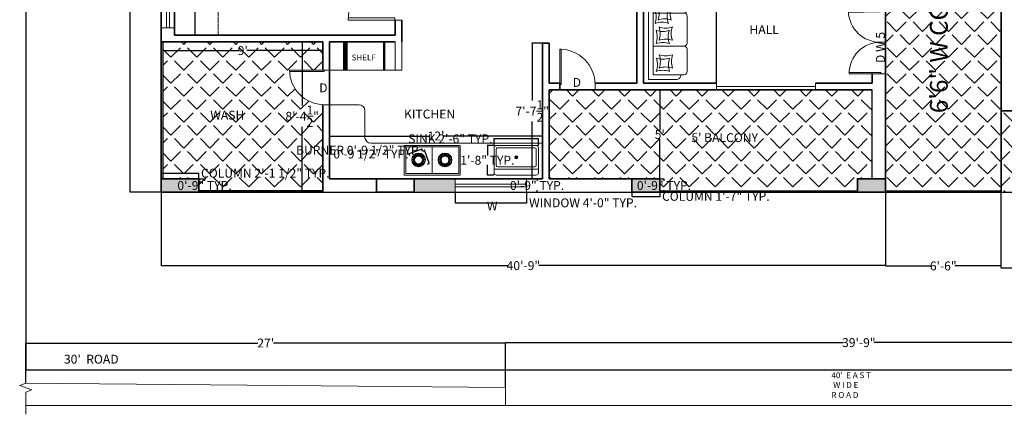
# Model space of a CAD drawing. Units: inches. Extents: x -2181 to 1225, y -80 to 4016.
# Tile 1 of 10: x 3 to 668, y -14 to 253. Entities that reach past the tile are written whole.
import ezdxf

# ---------------------------------------------------------------- set-up
doc = ezdxf.new("R2010")
doc.units = ezdxf.units.IN
doc.header["$MEASUREMENT"] = 0
doc.linetypes.add('ACAD_ISO02W100', pattern=[15, 12, -3])
for name, color, linetype, lineweight in [('A-ANNO-DIMS', 2, 'Continuous', 18), ('A-ANNO-TEXT', 7, 'Continuous', 18), ('A-AREA-IDEN', 7, 'Continuous', 18), ('A-COLS', 7, 'Continuous', 35), ('A-COLS-PATT', 252, 'Continuous', 13), ('A-DOOR', 3, 'Continuous', 18), ('A-EQPM', 9, 'Continuous', 18), ('A-FLOR', 7, 'Continuous', 25), ('A-FLOR-FIXT', 8, 'Continuous', 18), ('A-FLOR-PATT', 252, 'Continuous', 13), ('A-FURN', 30, 'Continuous', 18), ('A-GLAZ', 4, 'Continuous', 18), ('A-MILL', 8, 'Continuous', 18), ('A-MILL-OVHD', 8, 'ACAD_ISO02W100', 13), ('A-MILL-PATT', 252, 'Continuous', 13), ('A-WALL', 7, 'Continuous', 35), ('C-PROP', 7, 'Continuous', 30), ('C-ROAD', 8, 'Continuous', 18)]:
    doc.layers.add(name, color=color, linetype=linetype, lineweight=lineweight)
doc.styles.get("Standard").update_dxf_attribs({"font": 'arial.ttf'})
doc.dimstyles.get("Standard").update_dxf_attribs({"dimtxt": 6, "dimasz": 0.18, "dimexe": 0.18, "dimexo": 0.0625, "dimgap": 0.09, "dimtad": 0, "dimtih": 1, "dimtoh": 1, "dimdec": 4, "dimzin": 0, "dimdsep": 46, "dimlunit": 4, "dimtxsty": 'Standard', "dimcen": 0.09, "dimadec": 0, "dimazin": 0, "dimtfac": 1, "dimtdec": 4, "dimtofl": 0, "dimtmove": 0, "dimatfit": 3, "dimfxl": 1, "dimtolj": 1, "dimtzin": 0, "dimarcsym": 0})
pattern_1 = [(45, (0, 0), (-8.75045, 8.75045), [9, -3.375]), (135, (0, 0), (-8.75045, -8.75045), [9, -3.375])]

# ---------------------------------------------------------------- blocks, each defined once
blk = doc.blocks.new('*U2')
for p, q in [((0, 0), (0, -6)), ((40, 0), (40, -6))]:
    blk.add_line(p, q)
blk.add_lwpolyline([(0, 0), (0, 40), (1.75, 40), (1.75, 0)], close=True)
blk.add_arc((0, 0), 40, 0, 90)
blk = doc.blocks.new('Sink-single - 30 in top')
blk.add_line((-15, -3.999996), (15, -3.999996))
for points in [[(-13.5, 0), (13.5, 0)], [(-15, -18.499996), (-15, -1.5)], [(-13.5, -17.499996), (-13.5, -6.499996)], [(-12.5, -5.499996), (12.5, -5.499996)], [(13.5, -6.499996), (13.5, -17.499996)], [(15, -1.5), (15, -18.499996)], [(12.5, -18.499996), (-12.5, -18.499996)], [(13.5, -19.999996), (-13.5, -19.999996)]]:
    blk.add_lwpolyline(points)
for radius in [1, 0.5]:
    blk.add_circle((0, -11.999996), radius)
for centre, radius, start, end in [((-13.5, -1.5), 1.5, 90, 180), ((-12.5, -6.499996), 1, 90, 180), ((12.5, -6.499996), 1, 0, 90), ((13.5, -1.5), 1.5, 0, 90), ((-13.5, -18.499996), 1.5, 180, 270), ((-12.5, -17.499996), 1, 180, 270), ((12.5, -17.499996), 1, 270, 0), ((13.5, -18.499996), 1.5, 270, 0)]:
    blk.add_arc(centre, radius, start, end)
blk = doc.blocks.new('*D37')
at = {"layer": 'A-ANNO-DIMS', "color": 0, "lineweight": -2, "transparency": 16777216}
for p, q in [((107.58, 368.48), (121.67, 368.48)), ((121.49, 368.3), (121.49, 308.64)), ((121.49, 242.66), (121.49, 302.33)), ((107.58, 242.48), (121.67, 242.48))]:
    blk.add_line(p, q, dxfattribs=at)
at = {"layer": 'A-ANNO-DIMS', "color": 0, "transparency": 16777216}
for points in [[(121.46, 368.3), (121.52, 368.3), (121.49, 368.48)], [(121.46, 242.66), (121.52, 242.66), (121.49, 242.48)]]:
    blk.add_solid(points, dxfattribs=at)
at = {"layer": 'Defpoints', "color": 0, "transparency": 16777216}
for p in [(107.51, 368.48), (121.49, 368.48), (107.51, 242.48)]:
    blk.add_point(p, dxfattribs=at)
at = {"layer": 'A-ANNO-DIMS', "color": 0, "transparency": 16777216, "insert": (121.49, 305.48), "char_height": 6, "attachment_point": 5}
blk.add_mtext('\\A1;10\'-6"', dxfattribs=at)
blk = doc.blocks.new('*D38')
at = {"layer": 'A-ANNO-DIMS', "color": 0, "lineweight": -2, "transparency": 16777216}
for p, q in [((99.51, 237.92), (99.51, 231.91)), ((207.51, 237.92), (207.51, 231.91)), ((99.69, 232.09), (150.66, 232.09)), ((207.33, 232.09), (156.37, 232.09))]:
    blk.add_line(p, q, dxfattribs=at)
at = {"layer": 'A-ANNO-DIMS', "color": 0, "transparency": 16777216}
for points in [[(99.69, 232.12), (99.69, 232.06), (99.51, 232.09)], [(207.33, 232.12), (207.33, 232.06), (207.51, 232.09)]]:
    blk.add_solid(points, dxfattribs=at)
at = {"layer": 'Defpoints', "color": 0, "transparency": 16777216}
for p in [(99.51, 237.98), (207.51, 237.98), (207.51, 232.09)]:
    blk.add_point(p, dxfattribs=at)
at = {"layer": 'A-ANNO-DIMS', "color": 0, "transparency": 16777216, "insert": (153.51, 232.09), "char_height": 6, "attachment_point": 5}
blk.add_mtext("\\A1;9'", dxfattribs=at)
blk = doc.blocks.new('*D39')
at = {"layer": 'A-ANNO-DIMS', "color": 0, "lineweight": -2, "transparency": 16777216}
for p, q in [((207.45, 237.98), (193.47, 237.98)), ((193.65, 237.8), (193.65, 194.9)), ((193.65, 137.66), (193.65, 180.57)), ((207.45, 137.48), (193.47, 137.48))]:
    blk.add_line(p, q, dxfattribs=at)
at = {"layer": 'A-ANNO-DIMS', "color": 0, "transparency": 16777216}
for points in [[(193.62, 237.8), (193.68, 237.8), (193.65, 237.98)], [(193.62, 137.66), (193.68, 137.66), (193.65, 137.48)]]:
    blk.add_solid(points, dxfattribs=at)
at = {"layer": 'Defpoints', "color": 0, "transparency": 16777216}
for p in [(193.65, 237.98), (207.51, 237.98), (207.51, 137.48)]:
    blk.add_point(p, dxfattribs=at)
at = {"layer": 'A-ANNO-DIMS', "color": 0, "transparency": 16777216, "insert": (193.65, 187.73), "char_height": 6, "attachment_point": 5}
blk.add_mtext('\\A1;8\'-4{\\H1x;\\S1/2;}"', dxfattribs=at)
blk = doc.blocks.new('*D40')
at = {"layer": 'A-ANNO-DIMS', "color": 0, "lineweight": -2, "transparency": 16777216}
for p, q in [((212.01, 145.55), (212.01, 174.56)), ((212.19, 174.38), (279.12, 174.38)), ((355.83, 174.38), (288.91, 174.38)), ((356.01, 145.55), (356.01, 174.56))]:
    blk.add_line(p, q, dxfattribs=at)
at = {"layer": 'A-ANNO-DIMS', "color": 0, "transparency": 16777216}
for points in [[(212.19, 174.41), (212.19, 174.35), (212.01, 174.38)], [(355.83, 174.41), (355.83, 174.35), (356.01, 174.38)]]:
    blk.add_solid(points, dxfattribs=at)
at = {"layer": 'Defpoints', "color": 0, "transparency": 16777216}
for p in [(356.01, 174.38), (212.01, 145.48), (356.01, 145.48)]:
    blk.add_point(p, dxfattribs=at)
at = {"layer": 'A-ANNO-DIMS', "color": 0, "transparency": 16777216, "insert": (284.01, 174.38), "char_height": 6, "attachment_point": 5}
blk.add_mtext("\\A1;12'", dxfattribs=at)
blk = doc.blocks.new('*D41')
at = {"layer": 'A-ANNO-DIMS', "color": 0, "lineweight": -2, "transparency": 16777216}
for p, q in [((355.95, 236.98), (348.81, 236.98)), ((348.99, 236.8), (348.99, 198.35)), ((348.99, 145.66), (348.99, 184.12)), ((355.95, 145.48), (348.81, 145.48))]:
    blk.add_line(p, q, dxfattribs=at)
at = {"layer": 'A-ANNO-DIMS', "color": 0, "transparency": 16777216}
for points in [[(348.96, 236.8), (349.02, 236.8), (348.99, 236.98)], [(348.96, 145.66), (349.02, 145.66), (348.99, 145.48)]]:
    blk.add_solid(points, dxfattribs=at)
at = {"layer": 'Defpoints', "color": 0, "transparency": 16777216}
for p in [(356.01, 236.98), (348.99, 145.48), (356.01, 145.48)]:
    blk.add_point(p, dxfattribs=at)
at = {"layer": 'A-ANNO-DIMS', "color": 0, "transparency": 16777216, "insert": (348.99, 191.23), "char_height": 6, "attachment_point": 5}
blk.add_mtext('\\A1;7\'-7{\\H1x;\\S1/2;}"', dxfattribs=at)
blk = doc.blocks.new('*D42')
at = {"layer": 'A-ANNO-DIMS', "color": 0, "lineweight": -2, "transparency": 16777216}
for p, q in [((435.1, 205.3), (435.1, 178.63)), ((435.17, 205.48), (435.28, 205.48)), ((435.1, 145.66), (435.1, 172.34)), ((435.17, 145.48), (435.28, 145.48))]:
    blk.add_line(p, q, dxfattribs=at)
at = {"layer": 'A-ANNO-DIMS', "color": 0, "transparency": 16777216}
for points in [[(435.07, 205.3), (435.13, 205.3), (435.1, 205.48)], [(435.07, 145.66), (435.13, 145.66), (435.1, 145.48)]]:
    blk.add_solid(points, dxfattribs=at)
at = {"layer": 'Defpoints', "color": 0, "transparency": 16777216}
for p in [(435.1, 205.48), (435.1, 205.48), (435.1, 145.48)]:
    blk.add_point(p, dxfattribs=at)
at = {"layer": 'A-ANNO-DIMS', "color": 0, "transparency": 16777216, "insert": (435.1, 175.48), "char_height": 6, "attachment_point": 5}
blk.add_mtext("\\A1;5'", dxfattribs=at)
blk = doc.blocks.new('*D44')
at = {"layer": 'A-ANNO-DIMS', "color": 0, "lineweight": -2, "transparency": 16777216}
for p, q in [((473.37, 352.48), (473.48, 352.48)), ((473.3, 352.3), (473.3, 288.4)), ((473.3, 210.16), (473.3, 274.07)), ((473.37, 209.98), (473.48, 209.98))]:
    blk.add_line(p, q, dxfattribs=at)
at = {"layer": 'A-ANNO-DIMS', "color": 0, "transparency": 16777216}
for points in [[(473.27, 352.3), (473.33, 352.3), (473.3, 352.48)], [(473.27, 210.16), (473.33, 210.16), (473.3, 209.98)]]:
    blk.add_solid(points, dxfattribs=at)
at = {"layer": 'Defpoints', "color": 0, "transparency": 16777216}
for p in [(473.3, 352.48), (473.3, 352.48), (473.3, 209.98)]:
    blk.add_point(p, dxfattribs=at)
at = {"layer": 'A-ANNO-DIMS', "color": 0, "transparency": 16777216, "insert": (473.3, 281.23), "char_height": 6, "attachment_point": 5}
blk.add_mtext('\\A1;11\'-10{\\H1x;\\S1/2;}"', dxfattribs=at)
blk = doc.blocks.new('*D59')
at = {"layer": 'A-ANNO-DIMS', "color": 0, "lineweight": -2, "transparency": 16777216}
for p, q in [((587.51, 136.42), (587.51, 86.48)), ((665.51, 136.42), (665.51, 86.48)), ((587.69, 86.66), (618.43, 86.66)), ((665.33, 86.66), (634.6, 86.66))]:
    blk.add_line(p, q, dxfattribs=at)
at = {"layer": 'A-ANNO-DIMS', "color": 0, "transparency": 16777216}
for points in [[(587.69, 86.69), (587.69, 86.63), (587.51, 86.66)], [(665.33, 86.69), (665.33, 86.63), (665.51, 86.66)]]:
    blk.add_solid(points, dxfattribs=at)
at = {"layer": 'Defpoints', "color": 0, "transparency": 16777216}
for p in [(587.51, 136.48), (665.51, 136.48), (665.51, 86.66)]:
    blk.add_point(p, dxfattribs=at)
at = {"layer": 'A-ANNO-DIMS', "color": 0, "transparency": 16777216, "insert": (626.51, 86.66), "char_height": 6, "attachment_point": 5}
blk.add_mtext('\\A1;6\'-6"', dxfattribs=at)
blk = doc.blocks.new('*D60')
at = {"layer": 'A-ANNO-DIMS', "color": 0, "lineweight": -2, "transparency": 16777216}
for p, q in [((665.51, 136.42), (665.51, 85.31)), ((995.51, 136.42), (995.51, 85.31)), ((665.69, 85.49), (820.07, 85.49)), ((995.33, 85.49), (840.96, 85.49))]:
    blk.add_line(p, q, dxfattribs=at)
at = {"layer": 'A-ANNO-DIMS', "color": 0, "transparency": 16777216}
for points in [[(665.69, 85.52), (665.69, 85.46), (665.51, 85.49)], [(995.33, 85.52), (995.33, 85.46), (995.51, 85.49)]]:
    blk.add_solid(points, dxfattribs=at)
at = {"layer": 'Defpoints', "color": 0, "transparency": 16777216}
for p in [(665.51, 136.48), (995.51, 136.48), (995.51, 85.49)]:
    blk.add_point(p, dxfattribs=at)
at = {"layer": 'A-ANNO-DIMS', "color": 0, "transparency": 16777216, "insert": (830.51, 85.49), "char_height": 6, "attachment_point": 5}
blk.add_mtext('\\A1;27\'-6"', dxfattribs=at)
blk = doc.blocks.new('*D61')
at = {"layer": 'A-ANNO-DIMS', "color": 0, "lineweight": -2, "transparency": 16777216}
for p, q in [((98.51, 137.42), (98.51, 86.7)), ((587.51, 137.42), (587.51, 86.7)), ((98.69, 86.88), (332.5, 86.88)), ((587.33, 86.88), (353.53, 86.88))]:
    blk.add_line(p, q, dxfattribs=at)
at = {"layer": 'A-ANNO-DIMS', "color": 0, "transparency": 16777216}
for points in [[(98.69, 86.91), (98.69, 86.85), (98.51, 86.88)], [(587.33, 86.91), (587.33, 86.85), (587.51, 86.88)]]:
    blk.add_solid(points, dxfattribs=at)
at = {"layer": 'Defpoints', "color": 0, "transparency": 16777216}
for p in [(98.51, 137.48), (587.51, 137.48), (98.51, 86.88)]:
    blk.add_point(p, dxfattribs=at)
at = {"layer": 'A-ANNO-DIMS', "color": 0, "transparency": 16777216, "insert": (343.01, 86.88), "char_height": 6, "attachment_point": 5}
blk.add_mtext('\\A1;40\'-9"', dxfattribs=at)
blk = doc.blocks.new('*D67')
at = {"layer": 'A-ANNO-DIMS', "color": 0, "lineweight": -2, "transparency": 16777216}
for p, q in [((7.01, 7.55), (7.01, 34.78)), ((7.19, 34.6), (163.78, 34.6)), ((330.83, 34.6), (174.25, 34.6)), ((331.01, 4.55), (331.01, 34.78))]:
    blk.add_line(p, q, dxfattribs=at)
at = {"layer": 'A-ANNO-DIMS', "color": 0, "transparency": 16777216}
for points in [[(7.19, 34.63), (7.19, 34.57), (7.01, 34.6)], [(330.83, 34.63), (330.83, 34.57), (331.01, 34.6)]]:
    blk.add_solid(points, dxfattribs=at)
at = {"layer": 'Defpoints', "color": 0, "transparency": 16777216}
for p in [(331.01, 34.6), (7.01, 7.48), (331.01, 4.48)]:
    blk.add_point(p, dxfattribs=at)
at = {"layer": 'A-ANNO-DIMS', "color": 0, "transparency": 16777216, "insert": (169.01, 34.6), "char_height": 6, "attachment_point": 5}
blk.add_mtext("\\A1;27'", dxfattribs=at)
blk = doc.blocks.new('*D68')
at = {"layer": 'A-ANNO-DIMS', "color": 0, "lineweight": -2, "transparency": 16777216}
for p, q in [((331.01, 4.55), (331.01, 35.07)), ((331.19, 34.89), (559.12, 34.89)), ((807.83, 34.89), (579.91, 34.89)), ((808.01, 4.55), (808.01, 35.07))]:
    blk.add_line(p, q, dxfattribs=at)
at = {"layer": 'A-ANNO-DIMS', "color": 0, "transparency": 16777216}
for points in [[(331.19, 34.92), (331.19, 34.86), (331.01, 34.89)], [(807.83, 34.92), (807.83, 34.86), (808.01, 34.89)]]:
    blk.add_solid(points, dxfattribs=at)
at = {"layer": 'Defpoints', "color": 0, "transparency": 16777216}
for p in [(808.01, 34.89), (331.01, 4.48), (808.01, 4.48)]:
    blk.add_point(p, dxfattribs=at)
at = {"layer": 'A-ANNO-DIMS', "color": 0, "transparency": 16777216, "insert": (569.51, 34.89), "char_height": 6, "attachment_point": 5}
blk.add_mtext('\\A1;39\'-9"', dxfattribs=at)
blk = doc.blocks.new('*D72')
at = {"layer": 'A-ANNO-DIMS', "color": 0, "lineweight": -2, "transparency": 16777216}
for p, q in [((98.45, 572.98), (77.28, 572.98)), ((77.46, 572.8), (77.46, 361.9)), ((77.46, 136.66), (77.46, 347.57)), ((98.45, 136.48), (77.28, 136.48))]:
    blk.add_line(p, q, dxfattribs=at)
at = {"layer": 'A-ANNO-DIMS', "color": 0, "transparency": 16777216}
for points in [[(77.43, 572.8), (77.49, 572.8), (77.46, 572.98)], [(77.43, 136.66), (77.49, 136.66), (77.46, 136.48)]]:
    blk.add_solid(points, dxfattribs=at)
at = {"layer": 'Defpoints', "color": 0, "transparency": 16777216}
for p in [(77.46, 572.98), (98.51, 572.98), (98.51, 136.48)]:
    blk.add_point(p, dxfattribs=at)
at = {"layer": 'A-ANNO-DIMS', "color": 0, "transparency": 16777216, "insert": (77.46, 354.73), "char_height": 6, "attachment_point": 5}
blk.add_mtext('\\A1;36\'-4{\\H1x;\\S1/2;}"', dxfattribs=at)
blk = doc.blocks.new('SOFA-UPHOLSTERED')
for p, q in [((3.23, 44.91), (24.04, 44.91)), ((3.23, 22.57), (24.04, 22.58)), ((25.11, 22.58), (25.11, 22.58))]:
    blk.add_line(p, q)
for points in [[(0, 0), (0, 66.42), (18.76, 66.42, -0.414214), (20.91, 64.27), (20.91, 63.19)], [(3.23, 3.23), (3.23, 63.19), (24.21, 63.19, -0.417877), (26.36, 61.02), (26.19, 47.04, -0.410559), (24.04, 44.91), (3.23, 44.91)], [(26.19, 42.76), (26.19, 24.73, -0.414214), (24.04, 22.58), (3.23, 22.58)], [(26.19, 20.43), (26.19, 5.38, -0.414214), (24.04, 3.23), (3.23, 3.23)], [(21.99, 3.23), (21.99, 3.23, -0.414214), (18.76, 0), (0, 0)]]:
    blk.add_lwpolyline(points, format="xyb")
for points in [[(18.76, 66.42), (19, 66.42)], [(19, 0), (18.76, 0)]]:
    blk.add_lwpolyline(points)
for centre, radius, start, end in [((11.03, 74.56), 13.33, 250.26634, 289.73366), ((-6.02, 57.51), 13.33, 340.26634, 19.73366), ((28.07, 57.51), 13.33, 160.26634, 199.73366), ((9.03, 72.31), 13.33, 250.26634, 289.73366), ((-8.02, 55.27), 13.33, 340.26634, 19.73366), ((11.03, 40.47), 13.33, 70.26634, 109.73366), ((26.07, 55.27), 13.33, 160.26634, 199.73366), ((9.03, 38.22), 13.33, 70.26634, 109.73366), ((9.03, 59.47), 13.33, 250.26634, 289.73366), ((-8.02, 42.42), 13.33, 340.26634, 19.73366), ((11.03, 61.71), 13.33, 250.26634, 289.73366), ((-6.02, 44.66), 13.33, 340.26634, 19.73366), ((26.07, 42.42), 13.33, 160.26634, 199.73366), ((28.07, 44.66), 13.33, 160.26634, 199.73366), ((11.03, 27.62), 13.33, 70.26634, 109.73366), ((24.04, 42.76), 2.15, 360, 90), ((9.03, 25.38), 13.33, 70.26634, 109.73366), ((9.72, 45.79), 13.33, 250.26634, 289.73366), ((-7.33, 28.74), 13.33, 340.26634, 19.73366), ((11.72, 48.03), 13.33, 250.26634, 289.73366), ((-5.33, 30.99), 13.33, 340.26634, 19.73366), ((26.76, 28.74), 13.33, 160.26634, 199.73366), ((28.76, 30.99), 13.33, 160.26634, 199.73366), ((11.72, 13.94), 13.33, 70.26634, 109.73366), ((9.72, 11.7), 13.33, 70.26634, 109.73366), ((24.04, 20.43), 2.15, 0, 90.0249), ((9.86, 27), 13.33, 250.26634, 289.73366), ((-7.19, 9.96), 13.33, 340.26634, 19.73366), ((11.86, 29.25), 13.33, 250.26634, 289.73366), ((-5.19, 12.2), 13.33, 340.26634, 19.73366), ((26.9, 9.96), 13.33, 160.26634, 199.73366), ((28.9, 12.2), 13.33, 160.26634, 199.73366), ((11.86, -4.84), 13.33, 70.26634, 109.73366), ((9.86, -7.09), 13.33, 70.26634, 109.73366)]:
    blk.add_arc(centre, radius, start, end)
blk = doc.blocks.new('COOKTOP-BURNER')
for p, q in [((2.36, 5.97), (0.62, 6.97)), ((2.62, 6.35), (1.09, 7.64)), ((2.95, 6.68), (1.66, 8.21)), ((3.32, 6.94), (2.32, 8.68)), ((3.74, 7.14), (3.06, 9.02)), ((4.19, 7.26), (3.84, 9.23)), ((4.65, 7.3), (4.65, 9.3)), ((5.11, 7.26), (5.46, 9.23)), ((5.56, 7.14), (6.24, 9.02)), ((5.97, 6.94), (6.97, 8.68)), ((6.35, 6.68), (7.64, 8.21)), ((6.68, 6.35), (8.21, 7.64)), ((6.94, 5.97), (8.68, 6.97)), ((2, 4.65), (0, 4.65)), ((2.04, 5.11), (0.07, 5.46)), ((2.04, 4.19), (0.07, 3.84)), ((2.16, 5.55), (0.28, 6.24)), ((2.16, 3.74), (0.28, 3.06)), ((2.36, 3.32), (0.62, 2.32)), ((2.62, 2.95), (1.09, 1.66)), ((2.95, 2.62), (1.66, 1.09)), ((3.32, 2.35), (2.32, 0.62)), ((3.74, 2.16), (3.06, 0.28)), ((4.19, 2.04), (3.84, 0.07)), ((4.65, 2), (4.65, 0)), ((5.11, 2.04), (5.46, 0.07)), ((5.56, 2.16), (6.24, 0.28)), ((5.97, 2.35), (6.97, 0.62)), ((6.35, 2.62), (7.64, 1.09)), ((6.68, 2.95), (8.21, 1.66)), ((6.94, 3.32), (8.68, 2.32)), ((7.14, 5.55), (9.02, 6.24)), ((7.14, 3.74), (9.02, 3.06)), ((7.26, 5.11), (9.23, 5.46)), ((7.26, 4.19), (9.23, 3.84)), ((7.3, 4.65), (9.3, 4.65))]:
    blk.add_line(p, q)
for radius in [4.65, 2.65, 2.65, 2.65, 2.65, 2.65, 2.65, 2.65, 2.65, 2.65, 2.65, 2.65, 2.65, 2.65, 2.65, 2.65, 2.65, 2.65, 2.65, 2.65, 2.65, 2.65, 2.65, 2.65, 2.65, 2.65, 2.65, 2.65, 2.65, 2.65, 2.65, 2.65, 2.65, 2.65, 2.65, 2.65, 2.65]:
    blk.add_circle((4.65, 4.65), radius)
blk = doc.blocks.new('COL-18.89X9')
blk.add_lwpolyline([(18.9, 9), (0, 9), (0, 0), (18.9, 0)], close=True)
blk = doc.blocks.new('COL-25.37X9')
blk.add_lwpolyline([(0, 9), (25.37, 9), (25.37, 0), (0, 0)], close=True)
blk = doc.blocks.new('WIN-48')
for p, q in [((0, 9), (0, 0)), ((48, 9), (48, 0)), ((0, 5.5), (48, 5.5)), ((0, 3.5), (48, 3.5))]:
    blk.add_line(p, q)
blk = doc.blocks.new('*D90')
at = {"layer": 'A-ANNO-DIMS', "color": 0, "lineweight": -2, "transparency": 16777216}
for p, q in [((323.19, 172.51), (323.01, 172.51)), ((323.19, 168.07), (323.19, 172.69)), ((353.01, 172.51), (323.37, 172.51)), ((353.19, 168.07), (353.19, 172.69))]:
    blk.add_line(p, q, dxfattribs=at)
at = {"layer": 'A-ANNO-DIMS', "color": 0, "transparency": 16777216}
for points in [[(323.37, 172.54), (323.37, 172.48), (323.19, 172.51)], [(353.01, 172.54), (353.01, 172.48), (353.19, 172.51)]]:
    blk.add_solid(points, dxfattribs=at)
at = {"layer": 'Defpoints', "color": 0, "transparency": 16777216}
for p in [(323.19, 172.51), (323.19, 168.01), (353.19, 168.01)]:
    blk.add_point(p, dxfattribs=at)
at = {"layer": 'A-ANNO-DIMS', "color": 0, "transparency": 16777216, "insert": (293.7, 172.51), "char_height": 6, "attachment_point": 5}
blk.add_mtext('\\A1;SINK 2\'-6" TYP.', dxfattribs=at)
blk = doc.blocks.new('*D91')
at = {"layer": 'A-ANNO-DIMS', "color": 0, "lineweight": -2, "transparency": 16777216}
for p, q in [((323.13, 168.01), (318.51, 168.01)), ((318.69, 167.83), (318.69, 161.16)), ((318.69, 148.19), (318.69, 154.85)), ((323.13, 148.01), (318.51, 148.01))]:
    blk.add_line(p, q, dxfattribs=at)
at = {"layer": 'A-ANNO-DIMS', "color": 0, "transparency": 16777216}
for points in [[(318.66, 167.83), (318.72, 167.83), (318.69, 168.01)], [(318.66, 148.19), (318.72, 148.19), (318.69, 148.01)]]:
    blk.add_solid(points, dxfattribs=at)
at = {"layer": 'Defpoints', "color": 0, "transparency": 16777216}
for p in [(323.19, 168.01), (318.69, 148.01), (323.19, 148.01)]:
    blk.add_point(p, dxfattribs=at)
at = {"layer": 'A-ANNO-DIMS', "color": 0, "transparency": 16777216, "insert": (318.69, 158.01), "char_height": 6, "attachment_point": 5}
blk.add_mtext('\\A1;1\'-8" TYP.', dxfattribs=at)
blk = doc.blocks.new('*D102')
at = {"layer": 'A-ANNO-DIMS', "color": 0, "lineweight": -2, "transparency": 16777216}
for p, q in [((416.21, 136.42), (416.21, 133.47)), ((416.39, 133.65), (434.92, 133.65)), ((435.1, 136.42), (435.1, 133.47)), ((435.1, 133.65), (435.28, 133.65))]:
    blk.add_line(p, q, dxfattribs=at)
at = {"layer": 'A-ANNO-DIMS', "color": 0, "transparency": 16777216}
for points in [[(416.39, 133.68), (416.39, 133.62), (416.21, 133.65)], [(434.92, 133.68), (434.92, 133.62), (435.1, 133.65)]]:
    blk.add_solid(points, dxfattribs=at)
at = {"layer": 'Defpoints', "color": 0, "transparency": 16777216}
for p in [(416.21, 136.48), (435.1, 136.48), (435.1, 133.65)]:
    blk.add_point(p, dxfattribs=at)
at = {"layer": 'A-ANNO-DIMS', "color": 0, "transparency": 16777216, "insert": (472.95, 133.65), "char_height": 6, "attachment_point": 5}
blk.add_mtext('\\A1;COLUMN 1\'-7" TYP.', dxfattribs=at)
blk = doc.blocks.new('*D103')
at = {"layer": 'A-ANNO-DIMS', "color": 0, "lineweight": -2, "transparency": 16777216}
for p, q in [((435.17, 145.48), (438.12, 145.48)), ((437.94, 145.3), (437.94, 144.14)), ((435.17, 136.48), (438.12, 136.48)), ((437.94, 136.66), (437.94, 137.83))]:
    blk.add_line(p, q, dxfattribs=at)
at = {"layer": 'A-ANNO-DIMS', "color": 0, "transparency": 16777216}
for points in [[(437.91, 145.3), (437.97, 145.3), (437.94, 145.48)], [(437.91, 136.66), (437.97, 136.66), (437.94, 136.48)]]:
    blk.add_solid(points, dxfattribs=at)
at = {"layer": 'Defpoints', "color": 0, "transparency": 16777216}
for p in [(435.1, 145.48), (437.94, 145.48), (435.1, 136.48)]:
    blk.add_point(p, dxfattribs=at)
at = {"layer": 'A-ANNO-DIMS', "color": 0, "transparency": 16777216, "insert": (437.94, 140.98), "char_height": 6, "attachment_point": 5}
blk.add_mtext('\\A1;0\'-9" TYP.', dxfattribs=at)
blk = doc.blocks.new('*D114')
at = {"layer": 'A-ANNO-DIMS', "color": 0, "lineweight": -2, "transparency": 16777216}
for p, q in [((275.06, 164.19), (276.48, 164.71)), ((276.25, 164.82), (276.07, 164.82)), ((276.31, 164.65), (276.25, 164.82)), ((279.43, 156.08), (276.38, 164.48)), ((278.24, 155.45), (279.66, 155.97))]:
    blk.add_line(p, q, dxfattribs=at)
at = {"layer": 'A-ANNO-DIMS', "color": 0, "transparency": 16777216}
for points in [[(276.4, 164.49), (276.35, 164.47), (276.31, 164.65)], [(279.46, 156.09), (279.4, 156.07), (279.49, 155.91)]]:
    blk.add_solid(points, dxfattribs=at)
at = {"layer": 'Defpoints', "color": 0, "transparency": 16777216}
for p in [(275, 164.17), (276.31, 164.65), (278.18, 155.43)]:
    blk.add_point(p, dxfattribs=at)
at = {"layer": 'A-ANNO-DIMS', "color": 0, "transparency": 16777216, "insert": (231.98, 164.82), "char_height": 6, "attachment_point": 5}
blk.add_mtext('\\A1;BURNER 0\'-9 1/2" TYP.', dxfattribs=at)
blk = doc.blocks.new('*D115')
at = {"layer": 'A-ANNO-DIMS', "color": 0, "lineweight": -2, "transparency": 16777216}
for p, q in [((265.62, 162.24), (265.44, 162.24)), ((265.79, 162.3), (265.62, 162.24)), ((266.24, 161.05), (265.73, 162.47)), ((274.36, 165.42), (265.96, 162.36)), ((274.98, 164.23), (274.46, 165.65))]:
    blk.add_line(p, q, dxfattribs=at)
at = {"layer": 'A-ANNO-DIMS', "color": 0, "transparency": 16777216}
for points in [[(265.95, 162.39), (265.97, 162.33), (265.79, 162.3)], [(274.35, 165.45), (274.37, 165.39), (274.53, 165.48)]]:
    blk.add_solid(points, dxfattribs=at)
at = {"layer": 'Defpoints', "color": 0, "transparency": 16777216}
for p in [(265.79, 162.3), (266.27, 160.99), (275, 164.17)]:
    blk.add_point(p, dxfattribs=at)
at = {"layer": 'A-ANNO-DIMS', "color": 0, "transparency": 16777216, "insert": (240.07, 162.24), "char_height": 6, "attachment_point": 5}
blk.add_mtext('\\A1;0\'-9 1/2" TYP.', dxfattribs=at)
blk = doc.blocks.new('*D120')
at = {"layer": 'A-ANNO-DIMS', "color": 0, "lineweight": -2, "transparency": 16777216}
for p, q in [((98.51, 145.55), (98.51, 149.47)), ((98.69, 149.29), (123.7, 149.29)), ((123.88, 145.55), (123.88, 149.47)), ((123.88, 149.29), (124.06, 149.29))]:
    blk.add_line(p, q, dxfattribs=at)
at = {"layer": 'A-ANNO-DIMS', "color": 0, "transparency": 16777216}
for points in [[(98.69, 149.32), (98.69, 149.26), (98.51, 149.29)], [(123.7, 149.32), (123.7, 149.26), (123.88, 149.29)]]:
    blk.add_solid(points, dxfattribs=at)
at = {"layer": 'Defpoints', "color": 0, "transparency": 16777216}
for p in [(123.88, 149.29), (98.51, 145.48), (123.88, 145.48)]:
    blk.add_point(p, dxfattribs=at)
at = {"layer": 'A-ANNO-DIMS', "color": 0, "transparency": 16777216, "insert": (168.72, 149.29), "char_height": 6, "attachment_point": 5}
blk.add_mtext('\\A1;COLUMN 2\'-1 1/2" TYP.', dxfattribs=at)
blk = doc.blocks.new('*D121')
at = {"layer": 'A-ANNO-DIMS', "color": 0, "lineweight": -2, "transparency": 16777216}
for p, q in [((123.94, 145.48), (127.87, 145.48)), ((127.69, 145.3), (127.69, 144.14)), ((123.94, 136.48), (127.87, 136.48)), ((127.69, 136.66), (127.69, 137.83))]:
    blk.add_line(p, q, dxfattribs=at)
at = {"layer": 'A-ANNO-DIMS', "color": 0, "transparency": 16777216}
for points in [[(127.66, 145.3), (127.72, 145.3), (127.69, 145.48)], [(127.66, 136.66), (127.72, 136.66), (127.69, 136.48)]]:
    blk.add_solid(points, dxfattribs=at)
at = {"layer": 'Defpoints', "color": 0, "transparency": 16777216}
for p in [(123.88, 145.48), (123.88, 136.48), (127.69, 136.48)]:
    blk.add_point(p, dxfattribs=at)
at = {"layer": 'A-ANNO-DIMS', "color": 0, "transparency": 16777216, "insert": (127.69, 140.98), "char_height": 6, "attachment_point": 5}
blk.add_mtext('\\A1;0\'-9" TYP.', dxfattribs=at)
blk = doc.blocks.new('*D124')
at = {"layer": 'A-ANNO-DIMS', "color": 0, "lineweight": -2, "transparency": 16777216}
for p, q in [((297.04, 136.42), (297.04, 129.1)), ((345.04, 136.42), (345.04, 129.1)), ((297.22, 129.28), (344.86, 129.28)), ((345.04, 129.28), (345.22, 129.28))]:
    blk.add_line(p, q, dxfattribs=at)
at = {"layer": 'A-ANNO-DIMS', "color": 0, "transparency": 16777216}
for points in [[(297.22, 129.31), (297.22, 129.25), (297.04, 129.28)], [(344.86, 129.31), (344.86, 129.25), (345.04, 129.28)]]:
    blk.add_solid(points, dxfattribs=at)
at = {"layer": 'Defpoints', "color": 0, "transparency": 16777216}
for p in [(297.04, 136.48), (345.04, 136.48), (345.04, 129.28)]:
    blk.add_point(p, dxfattribs=at)
at = {"layer": 'A-ANNO-DIMS', "color": 0, "transparency": 16777216, "insert": (383.27, 129.28), "char_height": 6, "attachment_point": 5}
blk.add_mtext('\\A1;WINDOW 4\'-0" TYP.', dxfattribs=at)
blk = doc.blocks.new('*D125')
at = {"layer": 'A-ANNO-DIMS', "color": 0, "lineweight": -2, "transparency": 16777216}
for p, q in [((345.1, 145.48), (352.42, 145.48)), ((352.24, 145.3), (352.24, 144.14)), ((345.1, 136.48), (352.42, 136.48)), ((352.24, 136.66), (352.24, 137.83))]:
    blk.add_line(p, q, dxfattribs=at)
at = {"layer": 'A-ANNO-DIMS', "color": 0, "transparency": 16777216}
for points in [[(352.21, 145.3), (352.27, 145.3), (352.24, 145.48)], [(352.21, 136.66), (352.27, 136.66), (352.24, 136.48)]]:
    blk.add_solid(points, dxfattribs=at)
at = {"layer": 'Defpoints', "color": 0, "transparency": 16777216}
for p in [(345.04, 145.48), (352.24, 145.48), (345.04, 136.48)]:
    blk.add_point(p, dxfattribs=at)
at = {"layer": 'A-ANNO-DIMS', "color": 0, "transparency": 16777216, "insert": (352.24, 140.98), "char_height": 6, "attachment_point": 5}
blk.add_mtext('\\A1;0\'-9" TYP.', dxfattribs=at)

msp = doc.modelspace()

# ---------------------------------------------------------------- hatches: boundary and pattern name
at = {"layer": 'A-COLS-PATT'}
h = msp.add_hatch(color=256, dxfattribs=at)
h.dxf.hatch_style = 1
h.paths.add_polyline_path([(269.21166, 145.48479), (269.21166, 136.48479), (297.04101, 136.48479), (297.04101, 145.48479)])
h.paths.add_polyline_path([(445.01461, 352.48479), (445.01461, 361.48479), (426.1199, 361.48479), (426.1199, 352.48479)])
h.paths.add_polyline_path([(587.51461, 352.48479), (587.51461, 361.48479), (568.6199, 361.48479), (568.6199, 352.48479)])
h.paths.add_polyline_path([(518.40498, 421.48479), (518.40498, 430.48479), (503.51461, 430.48479), (503.51461, 421.48479)])
h.paths.add_polyline_path([(587.51461, 421.48479), (587.51461, 430.48479), (572.5711, 430.48479), (572.5711, 421.48479)])
h = msp.add_hatch(color=256, dxfattribs=at)
h.dxf.hatch_style = 1
h.paths.add_polyline_path([(98.51461, 145.48479), (98.51461, 136.48479), (123.88018, 136.48479), (123.88018, 145.48479)])
h = msp.add_hatch(color=256, dxfattribs=at)
h.dxf.hatch_style = 1
h.paths.add_polyline_path([(587.51461, 145.48479), (568.6199, 145.48479), (568.6199, 136.48479), (587.51461, 136.48479)])
h.paths.add_polyline_path([(435.10412, 145.48479), (416.20941, 145.48479), (416.20941, 136.48479), (435.10412, 136.48479)])
at = {"layer": 'A-FLOR-PATT'}
h = msp.add_hatch(dxfattribs=at)
h.set_pattern_fill('ANGLE', color=256, scale=45, angle=45)
h.set_pattern_definition(pattern_1)
h.paths.add_polyline_path([(626.51461, 392.98479), (626.51461, 425.98479), (587.51461, 425.98479), (587.51461, 137.48479), (665.51461, 137.48479), (665.51461, 392.98479)])
h = msp.add_hatch(dxfattribs=at)
h.set_pattern_fill('ANGLE', color=256, scale=45, angle=45)
h.set_pattern_definition(pattern_1)
h.paths.add_polyline_path([(99.51461, 145.48479), (123.88018, 145.48479), (123.88018, 137.48479), (207.51461, 137.48479), (207.51461, 195.57212, -0.389216795), (185.12809, 217.92652), (185.10569, 217.92652), (185.10569, 218.95023), (207.51461, 218.95023), (207.51461, 237.98479), (99.51461, 237.98479)])
h = msp.add_hatch(dxfattribs=at)
h.set_pattern_fill('ANGLE', color=256, scale=45, angle=45)
h.set_pattern_definition(pattern_1)
h.paths.add_polyline_path([(568.6199, 137.48479), (568.6199, 145.48479), (578.51461, 145.48479), (578.51461, 205.48479), (367.53774, 205.48479), (360.51461, 205.48479), (360.51461, 145.48479), (435.10412, 145.48479), (435.10412, 137.48479)])
h = msp.add_hatch(dxfattribs=at)
h.set_pattern_fill('ANGLE', color=256, scale=45, angle=45)
h.set_pattern_definition(pattern_1)
h.paths.add_polyline_path([(665.51461, 191.48479), (665.51461, 136.48479), (674.51461, 136.48479), (674.51461, 137.48479), (994.51461, 137.48479), (994.51461, 191.48479)])
at = {"layer": 'A-MILL-PATT'}
h = msp.add_hatch(dxfattribs=at)
h.set_pattern_fill('ANSI31', color=256, scale=4, angle=45, style=0)
h.paths.add_polyline_path([(221.01461, 218.95023), (224.01461, 218.95023), (224.01461, 237.98479), (221.01461, 237.98479)])
h = msp.add_hatch(dxfattribs=at)
h.set_pattern_fill('ANSI31', color=256, scale=4, angle=45, style=0)
h.paths.add_polyline_path([(248.01461, 218.95023), (249.51461, 218.95023), (249.51461, 237.98479), (248.01461, 237.98479)])

# ---------------------------------------------------------------- linework, layer by layer
at = {"layer": 'A-COLS'}
msp.add_line((435.10412, 145.48479), (435.10412, 136.48479), dxfattribs=at)
at = {"layer": 'A-EQPM'}
for p, q in [((281.44486, 149.04076), (281.44486, 167.02397)), ((290.08851, 160.8609), (290.08851, 162.8609))]:
    msp.add_line(p, q, dxfattribs=at)
for points in [[(262.52488, 168.02397), (300.36483, 168.02397), (300.36483, 148.04076), (262.52488, 148.04076)], [(263.52488, 167.02397), (299.36483, 167.02397), (299.36483, 149.04076), (263.52488, 149.04076)]]:
    msp.add_lwpolyline(points, close=True, dxfattribs=at)
for radius in [4.64904, 2.64904]:
    msp.add_circle((290.08851, 158.21185), radius, dxfattribs=at)
at = {"layer": 'A-FLOR'}
for points in [[(99.51461, 237.98479), (99.51461, 145.48479)], [(578.51461, 145.48479), (578.51461, 205.48479)], [(98.51461, 136.48479), (995.51461, 136.48479)], [(207.51461, 137.48479), (123.88018, 137.48479)], [(123.88018, 137.48479), (207.51461, 137.48479)], [(435.10412, 137.48479), (568.6199, 137.48479)], [(587.51461, 137.48479), (665.51461, 137.48479)]]:
    msp.add_lwpolyline(points, dxfattribs=at)
at = {"layer": 'A-GLAZ'}
for p, q in [((102.01461, 247.37629), (102.01461, 293.2354)), ((104.01461, 247.37629), (104.01461, 293.2354)), ((107.51461, 247.37629), (98.51461, 247.37629)), ((473.30295, 209.98479), (473.30295, 205.48479)), ((473.30295, 207.73479), (540.24794, 207.73479)), ((540.24794, 209.98479), (540.24794, 205.48479))]:
    msp.add_line(p, q, dxfattribs=at)
at = {"layer": 'A-MILL'}
for p, q in [((256.51461, 237.98479), (256.51461, 218.95023)), ((261.01461, 237.98479), (261.01461, 218.95023)), ((207.51461, 218.95023), (261.01461, 218.95023))]:
    msp.add_line(p, q, dxfattribs=at)
msp.add_lwpolyline([(212.01461, 195.55117), (232.01461, 195.55117, -0.414213562), (236.01461, 191.55117), (236.01461, 173.48479, 0.414213562), (240.01461, 169.48479), (356.01461, 169.48479)], format="xyb", dxfattribs=at)
at = {"layer": 'A-MILL-OVHD', "ltscale": 0.1}
msp.add_line((136.8586, 295.2354), (136.8586, 242.48479), dxfattribs=at)
at = {"layer": 'A-WALL'}
for p, q in [((256.51461, 252.70556), (256.51461, 242.48479)), ((261.01461, 252.70556), (261.01461, 237.98479)), ((367.53774, 209.98479), (367.53774, 205.48479))]:
    msp.add_line(p, q, dxfattribs=at)
for points in [[(587.51461, 572.98479), (98.51461, 572.98479), (98.51461, 136.48479)], [(587.51461, 136.48479), (587.51461, 572.98479)], [(665.51461, 136.48479), (665.51461, 572.98479)], [(107.51461, 368.48479), (107.51461, 242.48479)], [(419.51461, 209.98479), (419.51461, 281.23479)], [(424.01461, 209.98479), (424.01461, 281.23479)], [(256.51461, 242.48479), (107.51461, 242.48479)], [(207.51461, 237.98479), (98.51461, 237.98479)], [(207.51461, 237.98479), (207.51461, 218.95023)], [(256.51461, 237.98479), (212.01461, 237.98479)], [(212.01461, 237.98479), (212.01461, 145.48479)], [(356.01461, 236.98479), (356.01461, 145.48479)], [(356.01461, 236.98479), (360.51461, 236.98479)], [(360.51461, 236.98479), (360.51461, 209.98479)], [(578.51461, 209.98479), (578.51461, 216.40629)], [(360.51461, 209.98479), (367.53774, 209.98479)], [(391.40152, 209.98479), (419.51461, 209.98479)], [(424.01461, 209.98479), (473.30295, 209.98479)], [(540.24794, 209.98479), (578.51461, 209.98479)], [(360.51461, 205.48479), (367.53774, 205.48479)], [(360.51461, 205.48479), (360.51461, 145.48479)], [(367.53774, 205.48479), (578.51461, 205.48479)], [(207.51461, 195.57212), (207.51461, 136.48479)], [(665.51461, 191.48479), (995.51461, 191.48479)], [(212.01461, 145.48479), (356.01461, 145.48479)], [(360.51461, 145.48479), (435.10412, 145.48479)]]:
    msp.add_lwpolyline(points, dxfattribs=at)
at = {"layer": 'C-PROP'}
for points in [[(1087.01461, 16.48479), (1087.01461, 664.48479), (7.01461, 664.48479), (7.01461, 16.48479)], [(7.01461, 16.48479), (1087.01461, 16.48479)]]:
    msp.add_lwpolyline(points, dxfattribs=at)
at = {"layer": 'C-ROAD'}
for q in [(7.01461, 7.48479), (331.01461, -7.51521)]:
    msp.add_line((331.01461, 4.48479), q, dxfattribs=at)
for points in [[(7.01461, 22.48479), (7.01461, 7.48479), (2.8934, 5.98479), (11.13583, 2.98479), (7.01461, 1.48479), (7.01461, -13.51521)], [(7.01461, -7.51521), (1087.01461, -7.51521)]]:
    msp.add_lwpolyline(points, dxfattribs=at)

# ---------------------------------------------------------------- block references
at = {"layer": 'A-COLS', "extrusion": (0, 0, -1), "zscale": -1, "rotation": 180}
msp.add_blockref('COL-25.37X9', (-98.51451, 145.48457), dxfattribs=at)
at = {"layer": 'A-COLS'}
for name, p in [('COL-25.37X9', (243.846, 136.485)), ('COL-18.89X9', (416.209, 136.485))]:
    msp.add_blockref(name, p, dxfattribs=at)
at = {"layer": 'A-COLS', "rotation": 180}
msp.add_blockref('COL-18.89X9', (587.51502, 145.48457), dxfattribs=at)
at = {"layer": 'A-DOOR', "xscale": 0.7876317507006553, "yscale": 0.7876317507006553, "zscale": 0.7876317507006553, "rotation": 90.00000000000003}
msp.add_blockref('*U2', (256.28882, 252.70556), dxfattribs=at)
at = {"layer": 'A-DOOR', "extrusion": (0, 0, -1)}
for p, xscale, yscale, zscale, rotation in [((-583.8736, 259.13512), 0.5349745226309166, 0.5349745226309166, -0.5349745226309166, 268.8437329844228), ((-584.30477, 216.40629), -0.5349745226309166, 0.5349745226309166, -0.5349745226309166, 270), ((-208.50475, 218.95023), 0.5849766441292635, 0.5849766441292635, -0.5849766441292635, 270)]:
    msp.add_blockref('*U2', p, dxfattribs=dict(at, xscale=xscale, yscale=yscale, zscale=zscale, rotation=rotation))
at = {"layer": 'A-DOOR', "xscale": 0.5974492544575059, "yscale": 0.5974492544575059, "zscale": 0.5974492544575059}
msp.add_blockref('*U2', (367.52108, 209.06948), dxfattribs=at)
at = {"layer": 'A-EQPM', "rotation": 109.9999999999964}
msp.add_blockref('COOKTOP-BURNER', (278.18302, 155.43289), dxfattribs=at)
at = {"layer": 'A-EQPM'}
msp.add_blockref('COOKTOP-BURNER', (285.39745, 153.563), dxfattribs=at)
at = {"layer": 'A-FLOR-FIXT', "rotation": 180}
msp.add_blockref('Sink-single - 30 in top', (338.18916, 148.00679), dxfattribs=at)
at = {"layer": 'A-FURN'}
msp.add_blockref('SOFA-UPHOLSTERED', (427.379, 212.534), dxfattribs=at)
at = {"layer": 'A-GLAZ'}
msp.add_blockref('WIN-48', (297.041, 136.485), dxfattribs=at)

# ---------------------------------------------------------------- texts
at = {"layer": 'A-ANNO-TEXT', "insert": (581.04772, 219.98732), "char_height": 6, "attachment_point": 1, "rotation": 90}
msp.add_mtext_dynamic_manual_height_columns('  D W 5', width=291.4178321, gutter_width=1, heights=[6.10232], dxfattribs=at)
at = {"layer": 'A-ANNO-TEXT', "attachment_point": 1}
for s, width, insert, char_height in [('SHELF', 9.9941289, (226.97113, 229.40575), 4), ('D', 291.4178321, (376.3024, 213.57812), 6), ('D', 291.4178321, (205.13776, 209.93532), 6), ('W', 291.4178321, (318.38545, 130.11282), 6), ("30'  ROAD", 291.4178321, (32.78891, 26.7025), 6), ("{\\H0.66667x;40'  E A S T\\P W I D E\\PR O A D}", 291.4178321, (550.97092, 14.86513), 6)]:
    msp.add_mtext_dynamic_manual_height_columns(s, width=width, gutter_width=1, heights=[0], dxfattribs=dict(at, insert=insert, char_height=char_height))
at = {"layer": 'A-AREA-IDEN', "insert": (617.54393, 189.77481), "char_height": 12, "attachment_point": 1, "rotation": 90}
msp.add_mtext_dynamic_manual_height_columns('6\'6" W CORRIDOR', width=291.4178321, gutter_width=1, heights=[0], dxfattribs=at)
at = {"layer": 'A-AREA-IDEN', "char_height": 6, "attachment_point": 1}
for s, insert in [('HALL', (495.67694, 249.22651)), ('WASH', (131.57492, 191.45498)), ('KITCHEN', (262.4125, 192.2154)), ("5' BALCONY", (456.41571, 176.27942))]:
    msp.add_mtext_dynamic_manual_height_columns(s, width=291.4178321, gutter_width=1, heights=[0], dxfattribs=dict(at, insert=insert))

# ---------------------------------------------------------------- dimensions: what is measured, and where the dimension line sits
at = {"layer": 'A-ANNO-DIMS'}
for base, p1, p2, picture, middle in [((77.46081, 572.98479), (98.51461, 136.48479), (98.51461, 572.98479), '*D72', (77.46081, 354.73479)), ((121.48843, 368.48479), (107.51461, 242.48479), (107.51461, 368.48479), '*D37', (121.48843, 305.48479)), ((473.30295, 352.48479), (473.30295, 209.98479), (473.30295, 352.48479), '*D44', (473.30295, 281.23479)), ((193.6482, 237.98479), (207.51461, 137.48479), (207.51461, 237.98479), '*D39', (193.6482, 187.73479)), ((348.99251, 145.48479), (356.01461, 236.98479), (356.01461, 145.48479), '*D41', (348.99251, 191.23479)), ((435.10412, 205.48479), (435.10412, 145.48479), (435.10412, 205.48479), '*D42', (435.10412, 175.48479))]:
    dim = msp.add_linear_dim(base=base, p1=p1, p2=p2, angle=90, dimstyle='Standard', override={"dimclrd": 0, "dimclre": 0, "dimclrt": 0}, dxfattribs=at)
    dim.commit()
    dim.dimension.update_dxf_attribs({"geometry": picture, "text_midpoint": middle})
for base, p1, p2, picture, middle in [((207.51461, 232.08993), (99.51461, 237.98479), (207.51461, 237.98479), '*D38', (153.51461, 232.08993)), ((356.01461, 174.37794), (212.01461, 145.48479), (356.01461, 145.48479), '*D40', (284.01461, 174.37794)), ((98.51461, 86.88236), (587.51461, 137.48479), (98.51461, 137.48479), '*D61', (343.01461, 86.88236)), ((665.51461, 86.66051), (587.51461, 136.48479), (665.51461, 136.48479), '*D59', (626.51461, 86.66051)), ((995.51461, 85.49081), (665.51461, 136.48479), (995.51461, 136.48479), '*D60', (830.51461, 85.49081)), ((331.01461, 34.60009), (7.01461, 7.48479), (331.01461, 4.48479), '*D67', (169.01461, 34.60009)), ((808.01461, 34.89043), (331.01461, 4.48479), (808.01461, 4.48479), '*D68', (569.51461, 34.89043))]:
    dim = msp.add_linear_dim(base=base, p1=p1, p2=p2, dimstyle='Standard', override={"dimclrd": 0, "dimclre": 0, "dimclrt": 0}, dxfattribs=at)
    dim.commit()
    dim.dimension.update_dxf_attribs({"geometry": picture, "text_midpoint": middle})
for base, p1, p2, angle, text, picture, middle in [((323.18916, 172.50678), (353.18916, 168.00678), (323.18916, 168.00678), 180, 'SINK <> TYP.', '*D90', (293.70088, 172.50678)), ((276.31356, 164.64761), (278.18309, 155.43325), (275.00296, 164.17059), 110, 'BURNER <> TYP.', '*D114', (231.97654, 164.81676)), ((265.7886, 162.30106), (275.00296, 164.17059), (266.26562, 160.99046), 200, '<> TYP.', '*D115', (240.07251, 162.2395)), ((318.68916, 148.00679), (323.18916, 168.00678), (323.18916, 148.00679), 270, '<> TYP.', '*D91', (318.68916, 158.00679)), ((127.68501, 136.48479), (123.88018, 145.48479), (123.88018, 136.48479), 270, '<> TYP.', '*D121', (127.68501, 140.98479)), ((352.24101, 145.48479), (345.04101, 136.48479), (345.04101, 145.48479), 90, '<> TYP.', '*D125', (352.24101, 140.98479)), ((437.93833, 145.48479), (435.10412, 136.48479), (435.10412, 145.48479), 90, '<> TYP.', '*D103', (437.93833, 140.98479))]:
    dim = msp.add_linear_dim(base=base, p1=p1, p2=p2, angle=angle, text=text, dimstyle='Standard', override={"dimdec": 1, "dimlfac": 1, "dimrnd": 0, "dimzin": 1, "dimdsep": 46, "dimlunit": 4, "dimfrac": 2}, dxfattribs=at)
    dim.commit()
    dim.dimension.update_dxf_attribs({"geometry": picture, "text_midpoint": middle})
for base, p1, p2, text, picture, middle in [((123.88018, 149.28962), (98.51461, 145.48479), (123.88018, 145.48479), 'COLUMN <> TYP.', '*D120', (168.71839, 149.28962)), ((435.10412, 133.65058), (416.20941, 136.48479), (435.10412, 136.48479), 'COLUMN <> TYP.', '*D102', (472.95188, 133.65058)), ((345.04101, 129.28479), (297.04101, 136.48479), (345.04101, 136.48479), 'WINDOW <> TYP.', '*D124', (383.2735, 129.28479))]:
    dim = msp.add_linear_dim(base=base, p1=p1, p2=p2, text=text, dimstyle='Standard', override={"dimdec": 1, "dimlfac": 1, "dimrnd": 0, "dimzin": 1, "dimdsep": 46, "dimlunit": 4, "dimfrac": 2}, dxfattribs=at)
    dim.commit()
    dim.dimension.update_dxf_attribs({"geometry": picture, "text_midpoint": middle})

doc.saveas('drawing.dxf')
